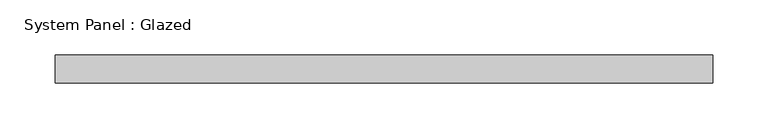
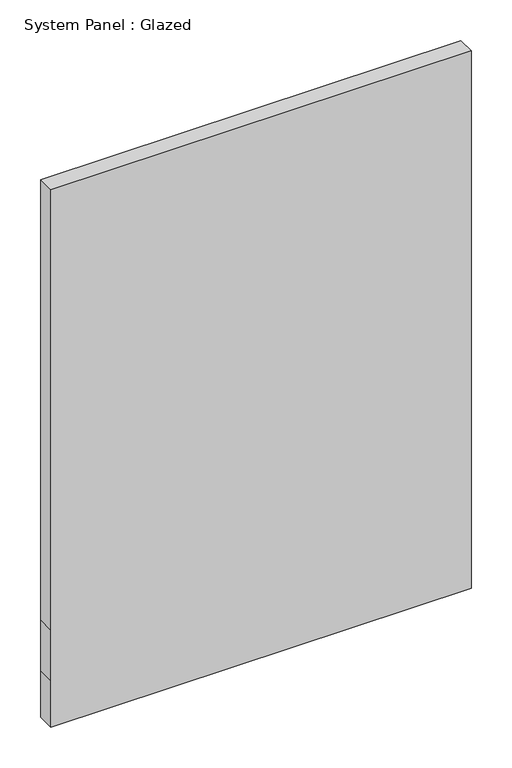
"""IFC4 building model written with IfcOpenShell, lengths in millimetres: plate geometry, System Panel : Glazed."""

from ifc_helpers import new_model, si_unit, frame, origin, place, context, project, spatial, polyline, outline, extrude, source, transform, mapped, element, save


def system_panel_glazed_d68d6f8b(model_context):
    return source(origin(), model_context, "Body", "SweptSolid", [
        extrude(outline(polyline([(0.0, -298.45), (0.0, 298.45), (69.85, 298.45), (146.05, 298.45), (807.2801773, 298.45), (807.2801773, -298.45), (146.05, -298.45), (69.85, -298.45), (0.0, -298.45)])), frame((0.0, 19.05, 0.0), z_axis=(0.0, 1.0, 0.0), x_axis=(0.0, 0.0, 1.0)), (0.0, 0.0, 1.0), 25.4),
    ])


if __name__ == "__main__":
    model = new_model("IFC4")
    model_context = context("Model", 3, world=origin())
    ifc_project = project(units=[si_unit("LENGTHUNIT", "METRE", prefix="MILLI")], contexts=[model_context])
    site = spatial("IfcSite", under=ifc_project)
    building = spatial("IfcBuilding", under=site)
    placement = place(None, origin())
    system_panel_glazed_shape = system_panel_glazed_d68d6f8b(model_context)
    element("IfcPlate", 1, ObjectType="System Panel : Glazed", at=placement, inside=building, context=model_context, shape_type="MappedRepresentation", body=[
        mapped(system_panel_glazed_shape, transform((0.0, 0.0, 0.0), x_axis=(1.0, 0.0, 0.0), y_axis=(0.0, 1.0, 0.0), z_axis=(0.0, 0.0, 1.0))),
    ])
    save(model, "model.ifc")

# Revit data of these elements
# Type "System Panel : Glazed"
#   Construction Type Id = "GSP4R"
#   Analytic Construction = "1/8 in Pilkington single glazing"
#   Visual Light Transmittance = 0.9
#   Solar Heat Gain Coefficient = 0.86
#   Heat Transfer Coefficient (U) = 1.18115 BTU/(h·ft²·°F)
#   Define Thermal Properties by = 1
# Element 1 (IfcPlate, "System Panel : Glazed")
#   Materials on its faces: "Glass"
# Materials
#   "Glass": class "Glass", colour RGB 0 128 192, transparency 0.75, Description = "Soda Lime Glass", Cost = 0
